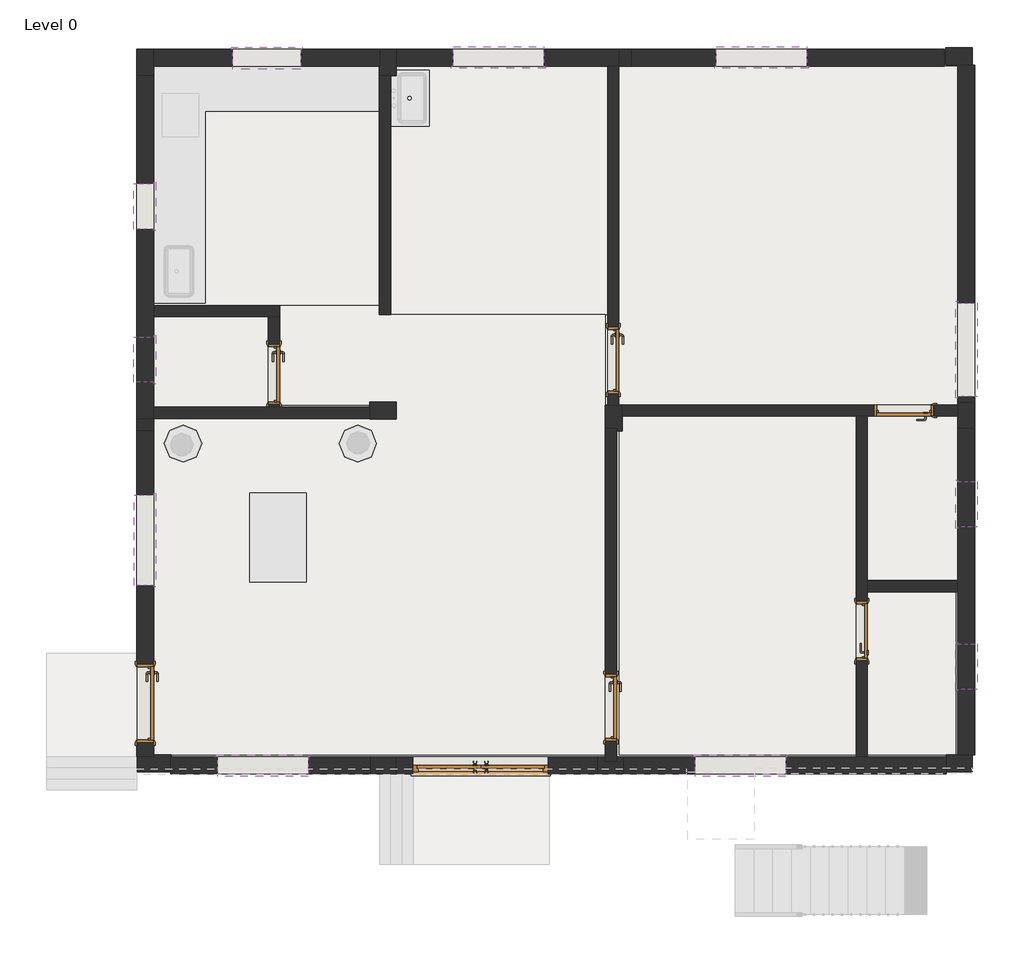
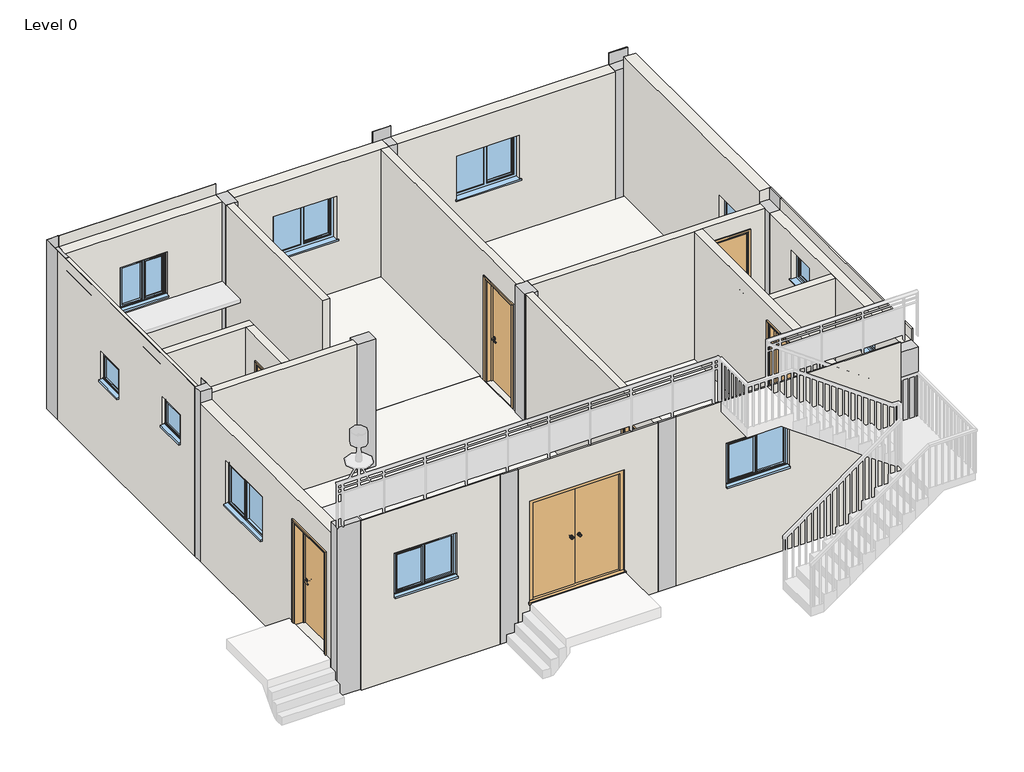
# One storey, part 1 of 3: 19 walls, 12 columns, 11 windows, 7 doors, 5 slabs.
# Revit data of these elements (continued)
# Type "Windows_Dbl_Plain : W3" (continued)
#   Height = 2.985564 ft
#   Width = 4.136 ft
#   Heat Transfer Coefficient (U) = 3.6886 W/(m²·K)
#   Glazing Thickness = 0.07874 ft
#   FrameOffset - External = 0.164042 ft
#   Frame Depth = 0.213255 ft
#   Default Head Height = 6.922572 ft
#   Cill Depth = 0.287073 ft
#   Cavity Closer Width = 0.164042 ft
#   Cavity Closer Offset from Ext = 0.336286 ft
#   Cavity Closer Depth = 0.278871 ft
#   Vis - Cavity Closers = yes
#   Define Thermal Properties by = 1
#   Material Trim = Window Frame
#   Material Glass = Glass
#   Material Frame = Cherry
#   Wall Closure = (empty or 0)
# Type "Windows_Dbl_Plain : W4"
#   Type Mark = "58"
#   Operation = "DoublePanelVertical"
#   Construction Type Id = "GSP4R"
#   Manufacturer = "Revit"
#   Keynote = "L10"
#   Analytic Construction = "1/8 in Pilkington single glazing"
#   Wrap Layers (Ext) from Ext = 0.336286 ft
#   Wrap Layers (Int) from Ext = 0.582349 ft
#   Window Board Projection = 0.082021 ft
#   Window Board Extension = 0.082021 ft
#   Visual Light Transmittance = 0.9
#   Solar Heat Gain Coefficient = 0.78
#   Rough Width = 4.0 ft
#   Rough Height = 2.985564 ft
#   Height = 2.985564 ft
#   Width = 4.0 ft
#   Heat Transfer Coefficient (U) = 3.6886 W/(m²·K)
#   Glazing Thickness = 0.07874 ft
#   FrameOffset - External = 0.164042 ft
#   Frame Depth = 0.213255 ft
#   Default Head Height = 6.922572 ft
#   Cill Depth = 0.287073 ft
#   Cavity Closer Width = 0.164042 ft
#   Cavity Closer Offset from Ext = 0.336286 ft
#   Cavity Closer Depth = 0.278871 ft
#   Vis - Cavity Closers = yes
#   Define Thermal Properties by = 1
#   Material Trim = Window Frame
#   Material Glass = Glass
#   Material Frame = Cherry
#   Wall Closure = (empty or 0)
# Type "Windows_Dbl_Plain : W5"
#   Type Mark = "57"
#   Operation = "DoublePanelVertical"
#   Construction Type Id = "GSP4R"
#   Manufacturer = "Revit"
#   Keynote = "L10"
#   Analytic Construction = "1/8 in Pilkington single glazing"
#   Wrap Layers (Ext) from Ext = 0.336286 ft
#   Wrap Layers (Int) from Ext = 0.582349 ft
#   Window Board Projection = 0.082021 ft
#   Window Board Extension = 0.082021 ft
#   Visual Light Transmittance = 0.9
#   Solar Heat Gain Coefficient = 0.78
#   Rough Width = 4.018 ft
#   Rough Height = 2.985564 ft
#   Height = 2.985564 ft
#   Width = 4.018 ft
#   Heat Transfer Coefficient (U) = 3.6886 W/(m²·K)
#   Glazing Thickness = 0.07874 ft
#   FrameOffset - External = 0.164042 ft
#   Frame Depth = 0.213255 ft
#   Default Head Height = 6.922572 ft
#   Cill Depth = 0.287073 ft
#   Cavity Closer Width = 0.164042 ft
#   Cavity Closer Offset from Ext = 0.336286 ft
#   Cavity Closer Depth = 0.278871 ft
#   Vis - Cavity Closers = yes
#   Define Thermal Properties by = 1
#   Material Trim = Window Frame
#   Material Glass = Glass
#   Material Frame = Cherry
#   Wall Closure = (empty or 0)
# Type "Windows_Dbl_Plain : W6"
#   Type Mark = "56"
#   Operation = "DoublePanelVertical"
#   Construction Type Id = "GSP4R"
#   Manufacturer = "Revit"
#   Keynote = "L10"
#   Analytic Construction = "1/8 in Pilkington single glazing"
#   Wrap Layers (Ext) from Ext = 0.336286 ft
#   Wrap Layers (Int) from Ext = 0.582349 ft
#   Window Board Projection = 0.082021 ft
#   Window Board Extension = 0.082021 ft
#   Visual Light Transmittance = 0.9
#   Solar Heat Gain Coefficient = 0.78
#   Rough Width = 3.0 ft
#   Rough Height = 2.985564 ft
#   Height = 2.985564 ft
#   Width = 3.0 ft
#   Heat Transfer Coefficient (U) = 3.6886 W/(m²·K)
#   Glazing Thickness = 0.07874 ft
#   FrameOffset - External = 0.164042 ft
#   Frame Depth = 0.213255 ft
#   Default Head Height = 6.922572 ft
#   Cill Depth = 0.287073 ft
#   Cavity Closer Width = 0.164042 ft
#   Cavity Closer Offset from Ext = 0.336286 ft
#   Cavity Closer Depth = 0.278871 ft
#   Vis - Cavity Closers = yes
#   Define Thermal Properties by = 1
#   Material Trim = Window Frame
#   Material Glass = Glass
#   Material Frame = Cherry
#   Wall Closure = (empty or 0)
# Type "Windows_Dbl_Plain : W7"
#   Type Mark = "63"
#   Operation = "DoublePanelVertical"
#   Construction Type Id = "GSP4R"
#   Manufacturer = "Revit"
#   Keynote = "L10"
#   Analytic Construction = "1/8 in Pilkington single glazing"
#   Wrap Layers (Ext) from Ext = 0.336286 ft
#   Wrap Layers (Int) from Ext = 0.582349 ft
#   Window Board Projection = 0.082021 ft
#   Window Board Extension = 0.082021 ft
#   Visual Light Transmittance = 0.9
#   Solar Heat Gain Coefficient = 0.78
#   Rough Width = 4.0 ft
#   Rough Height = 2.985564 ft
#   Height = 2.985564 ft
#   Width = 4.0 ft
#   Heat Transfer Coefficient (U) = 3.6886 W/(m²·K)
#   Glazing Thickness = 0.07874 ft
#   FrameOffset - External = 0.164042 ft
#   Frame Depth = 0.213255 ft
#   Default Head Height = 6.922572 ft
#   Cill Depth = 0.287073 ft
#   Cavity Closer Width = 0.164042 ft
#   Cavity Closer Offset from Ext = 0.336286 ft
#   Cavity Closer Depth = 0.278871 ft
#   Vis - Cavity Closers = yes
#   Define Thermal Properties by = 1
#   Material Trim = Window Frame
#   Material Glass = Glass
#   Material Frame = Cherry
#   Wall Closure = (empty or 0)
# Type "Windows_Dbl_Plain : WN"
#   Type Mark = "61"
#   Operation = "DoublePanelVertical"
#   Construction Type Id = "GSP4R"
#   Manufacturer = "Revit"
#   Keynote = "L10"
#   Analytic Construction = "1/8 in Pilkington single glazing"
#   Wrap Layers (Ext) from Ext = 0.336286 ft
#   Wrap Layers (Int) from Ext = 0.582349 ft
#   Window Board Projection = 0.082021 ft
#   Window Board Extension = 0.082021 ft
#   Visual Light Transmittance = 0.9
#   Solar Heat Gain Coefficient = 0.78
#   Rough Width = 4.0 ft
#   Rough Height = 2.985564 ft
#   Height = 2.985564 ft
#   Width = 4.0 ft
#   Heat Transfer Coefficient (U) = 3.6886 W/(m²·K)
#   Glazing Thickness = 0.07874 ft
#   FrameOffset - External = 0.164042 ft
#   Frame Depth = 0.213255 ft
#   Default Head Height = 6.922572 ft
#   Cill Depth = 0.287073 ft
#   Cavity Closer Width = 0.164042 ft
#   Cavity Closer Offset from Ext = 0.336286 ft
#   Cavity Closer Depth = 0.278871 ft
#   Vis - Cavity Closers = yes
#   Define Thermal Properties by = 1
#   Material Trim = Window Frame
#   Material Glass = Glass
#   Material Frame = Cherry
#   Wall Closure = (empty or 0)
# Type "Windows_Sgl_Plain : VW1"
#   Type Mark = "64"
#   Operation = "SinglePanel"
#   Construction Type Id = "SGL"
#   Manufacturer = "Revit"
#   Keynote = "L10"
#   Analytic Construction = "Large single-glazed windows"
#   Wrap Layers (Ext) from Ext = 0.336286 ft
#   Wrap Layers (Int) from Ext = 0.582349 ft
#   Window Board Projection = 0.082021 ft
#   Window Board Extension = 0.082021 ft
#   Visual Light Transmittance = 0.9
#   Solar Heat Gain Coefficient = 0.86
#   Rough Width = 2.0 ft
#   Rough Height = 2.0 ft
#   Height = 2.0 ft
#   Width = 2.0 ft
#   Heat Transfer Coefficient (U) = 5.5617 W/(m²·K)
#   Glazing Thickness = 0.07874 ft
#   FrameOffset - External = 0.164042 ft
#   Frame Depth = 0.213255 ft
#   Default Head Height = 6.922572 ft
#   Cill Depth = 0.287073 ft
#   Cavity Closer Width = 0.164042 ft
#   Cavity Closer Offset from Ext = 0.336286 ft
#   Cavity Closer Depth = 0.278871 ft
#   Vis - Cavity Closers = yes
#   Define Thermal Properties by = 1
#   Material Trim = Window Frame
#   Material Glass = Glass
#   Material Frame = Window Frame
#   Wall Closure = (empty or 0)
# Type "Windows_Sgl_Plain : VW2"
#   Type Mark = "65"
#   Operation = "SinglePanel"
#   Construction Type Id = "SGL"
#   Manufacturer = "Revit"
#   Keynote = "L10"
#   Analytic Construction = "Large single-glazed windows"
#   Wrap Layers (Ext) from Ext = 0.336286 ft
#   Wrap Layers (Int) from Ext = 0.582349 ft
#   Window Board Projection = 0.082021 ft
#   Window Board Extension = 0.082021 ft
#   Visual Light Transmittance = 0.9
#   Solar Heat Gain Coefficient = 0.86
#   Rough Width = 2.0 ft
#   Rough Height = 2.0 ft
#   Height = 2.0 ft
#   Width = 2.0 ft
#   Heat Transfer Coefficient (U) = 5.5617 W/(m²·K)
#   Glazing Thickness = 0.07874 ft
#   FrameOffset - External = 0.164042 ft
#   Frame Depth = 0.213255 ft
#   Default Head Height = 6.922572 ft
#   Cill Depth = 0.287073 ft
#   Cavity Closer Width = 0.164042 ft
#   Cavity Closer Offset from Ext = 0.336286 ft
#   Cavity Closer Depth = 0.278871 ft
#   Vis - Cavity Closers = yes
#   Define Thermal Properties by = 1
#   Material Trim = Window Frame
#   Material Glass = Glass
#   Material Frame = Window Frame
#   Wall Closure = (empty or 0)
# Type "Windows_Sgl_Plain : VW3"
#   Type Mark = "44"
#   Operation = "SinglePanel"
#   Construction Type Id = "SGL"
#   Manufacturer = "Revit"
#   Keynote = "L10"
#   Analytic Construction = "Large single-glazed windows"
#   Wrap Layers (Ext) from Ext = 0.336286 ft
#   Wrap Layers (Int) from Ext = 0.582349 ft
#   Window Board Projection = 0.082021 ft
#   Window Board Extension = 0.082021 ft
#   Visual Light Transmittance = 0.9
#   Solar Heat Gain Coefficient = 0.86
#   Rough Width = 2.0 ft
#   Rough Height = 2.0 ft
#   Height = 2.0 ft
#   Width = 2.0 ft
#   Heat Transfer Coefficient (U) = 5.5617 W/(m²·K)
#   Glazing Thickness = 0.07874 ft
#   FrameOffset - External = 0.164042 ft
#   Frame Depth = 0.213255 ft
#   Default Head Height = 6.922572 ft
#   Cill Depth = 0.287073 ft
#   Cavity Closer Width = 0.164042 ft
#   Cavity Closer Offset from Ext = 0.336286 ft
#   Cavity Closer Depth = 0.278871 ft
#   Vis - Cavity Closers = yes
#   Define Thermal Properties by = 1
#   Material Trim = Window Frame
#   Material Glass = Glass
#   Material Frame = Window Frame
#   Wall Closure = (empty or 0)
# Type "Windows_Sgl_Plain : VW4"
#   Type Mark = "60"
#   Operation = "SinglePanel"
#   Construction Type Id = "SGL"
#   Manufacturer = "Revit"
#   Keynote = "L10"
#   Analytic Construction = "Large single-glazed windows"
#   Wrap Layers (Ext) from Ext = 0.336286 ft
#   Wrap Layers (Int) from Ext = 0.582349 ft
#   Window Board Projection = 0.082021 ft
#   Window Board Extension = 0.082021 ft
#   Visual Light Transmittance = 0.9
#   Solar Heat Gain Coefficient = 0.86
#   Rough Width = 2.0 ft
#   Rough Height = 2.0 ft
#   Height = 2.0 ft
#   Width = 2.0 ft
#   Heat Transfer Coefficient (U) = 5.5617 W/(m²·K)
#   Glazing Thickness = 0.07874 ft
#   FrameOffset - External = 0.164042 ft
#   Frame Depth = 0.213255 ft
#   Default Head Height = 6.922572 ft
#   Cill Depth = 0.287073 ft
#   Cavity Closer Width = 0.164042 ft
#   Cavity Closer Offset from Ext = 0.336286 ft
#   Cavity Closer Depth = 0.278871 ft
#   Vis - Cavity Closers = yes
#   Define Thermal Properties by = 1
#   Material Trim = Window Frame
#   Material Glass = Glass
#   Material Frame = Window Frame
#   Wall Closure = (empty or 0)
# Elements 1, 2, 3, 4, 5, 6, 7, 8, 9 (IfcColumn, "Columns_Rectangular : C1")
#   Phase Created = New Construction
#   Materials on its faces: "Concrete, Precast"
# Elements 10, 11, 12 (IfcColumn, "Columns_Rectangular : C2")
#   Phase Created = New Construction
#   Materials on its faces: "Concrete, Precast"
# Element 13 (IfcDoor, "Doors_ExtDbl_Flush : D1")
#   Phase Created = New Construction
#   Materials on its faces: "Door - Handle", "Door - Frame/Mullion", "Door - Panel"
# Element 14 (IfcDoor, "Doors_IntSgl : D2")
#   Phase Created = New Construction
#   Materials on its faces: "Door - Architrave", "Door - Handle", "Door - Frame/Mullion (1)", "Door - Panel"
# Element 15 (IfcDoor, "Doors_IntSgl : D3")
#   Phase Created = New Construction
#   Materials on its faces: "Door - Architrave", "Door - Handle", "Door - Frame/Mullion (1)", "Door - Panel"
# Element 16 (IfcDoor, "Doors_IntSgl : D4")
#   Phase Created = New Construction
#   Materials on its faces: "Door - Architrave", "Door - Handle", "Door - Frame/Mullion (1)", "Door - Panel"
# Element 17 (IfcDoor, "Doors_IntSgl : D5")
#   Phase Created = New Construction
#   Materials on its faces: "Door - Architrave", "Door - Handle", "Door - Frame/Mullion (1)", "Door - Panel"
# Element 18 (IfcDoor, "Doors_IntSgl : D6")
#   Phase Created = New Construction
#   Materials on its faces: "Door - Architrave", "Door - Handle", "Door - Frame/Mullion (1)", "Door - Panel"
# Element 19 (IfcDoor, "Doors_IntSgl : D7")
#   Phase Created = New Construction
#   Materials on its faces: "Door - Architrave", "Door - Handle", "Door - Frame/Mullion (1)", "Door - Panel"
# Element 20 (IfcSlab)
#   Height Offset From Level = 0.492 ft
#   Phase Created = New Construction
#   Materials on its faces: "Structure, Timber Joist/Rafter Layer"
# Element 21 (IfcSlab, "BEDROOM FLOOR")
#   Height Offset From Level = 0.492 ft
#   Phase Created = New Construction
#   Materials on its faces: "Structure, Timber Joist/Rafter Layer", "BEDROOM FLOOR TEXTURE"
# Element 22 (IfcSlab, "KITCHEN FLOOR")
#   Height Offset From Level = 0.492 ft
#   Phase Created = New Construction
#   Materials on its faces: "Structure, Timber Joist/Rafter Layer", "KITCHEN FLOOR TEXTURE"
# Element 23 (IfcSlab, "LIVING ROOM")
#   built-in parameter 1001955 = 3.14159 (stored number, unit not read)
#   Height Offset From Level = 0.492 ft
#   Phase Created = New Construction
#   Materials on its faces: "Structure, Timber Joist/Rafter Layer", "LIVING ROOM FLOOR TEXTURE"
# Element 24 (IfcSlab, "TOILET FLOOR")
#   built-in parameter 1001955 = 3.14159 (stored number, unit not read)
#   Height Offset From Level = 0.984 ft
#   Phase Created = New Construction
#   Materials on its faces: "Structure, Timber Joist/Rafter Layer", "TOILET FLOOR TEXTURE"
# Elements 25, 26, 27, 28, 29, 30, 31, 32, 33, 34 (IfcWall, "EX WALL")
#   built-in parameter 1001111 = -1.551 ft
#   Top Offset = 0.0 ft
#   Base Offset = -1.551 ft
#   wall height = 11.39352 ft
#   Phase Created = New Construction
#   Base Constraint = Level 0
#   Top Constraint = Level 1
#   Materials on its faces: "Brick, Common"
# Elements 35, 36, 37, 38, 39, 40, 41, 42, 43 (IfcWall, "INNER WALL")
#   Top Offset = 0.0 ft
#   Base Offset = 0.0 ft
#   wall height = 9.84252 ft
#   Phase Created = New Construction
#   Base Constraint = Level 0
#   Top Constraint = Level 1
#   Materials on its faces: "Brick, Common"
# Element 44 (IfcWindow, "Windows_Dbl_Plain : W1")
#   Mark = "W1"
#   Phase Created = New Construction
#   Materials on its faces: "Cherry", "Glass", "Window Frame"
# Element 45 (IfcWindow, "Windows_Dbl_Plain : W3")
#   Mark = "W3"
#   Phase Created = New Construction
#   Materials on its faces: "Cherry", "Glass", "Window Frame"
# Element 46 (IfcWindow, "Windows_Dbl_Plain : W4")
#   Mark = "W4"
#   Phase Created = New Construction
#   Materials on its faces: "Cherry", "Glass", "Window Frame"
# Element 47 (IfcWindow, "Windows_Dbl_Plain : W5")
#   Mark = "W5"
#   Phase Created = New Construction
#   Materials on its faces: "Cherry", "Glass", "Window Frame"
# Element 48 (IfcWindow, "Windows_Dbl_Plain : W6")
#   Mark = "W6"
#   Phase Created = New Construction
#   Materials on its faces: "Cherry", "Glass", "Window Frame"
# Element 49 (IfcWindow, "Windows_Dbl_Plain : W7")
#   Mark = "W7"
#   Phase Created = New Construction
#   Materials on its faces: "Cherry", "Glass", "Window Frame"
# Element 50 (IfcWindow, "Windows_Dbl_Plain : WN")
#   Mark = "W2"
#   Phase Created = New Construction
#   Materials on its faces: "Cherry", "Glass", "Window Frame"
# Element 51 (IfcWindow, "Windows_Sgl_Plain : VW1")
#   Mark = "VW1"
#   Phase Created = New Construction
#   Materials on its faces: "Window Frame", "Glass"
# Element 52 (IfcWindow, "Windows_Sgl_Plain : VW2")
#   Mark = "VW2"
#   Phase Created = New Construction
#   Materials on its faces: "Window Frame", "Glass"
# Element 53 (IfcWindow, "Windows_Sgl_Plain : VW3")
#   Mark = "VW3"
#   Phase Created = New Construction
#   Materials on its faces: "Window Frame", "Glass"
# Element 54 (IfcWindow, "Windows_Sgl_Plain : VW4")
#   Mark = "VW4"
#   Phase Created = New Construction
#   Materials on its faces: "Window Frame", "Glass"
# Materials
#   "Concrete, Precast": class "Concrete", colour RGB 192 192 192, transparency 0, Description = "Precast concrete", Cost = 0
#   "Door - Panel": class "Wood", colour RGB 210 159 95, transparency 0, Keynote = "L20", Cost = 0
#   "Door - Frame/Mullion": class "Wood", colour RGB 212 179 113, transparency 0, Keynote = "L20", Cost = 0
#   "Door - Handle": colour RGB 0 0 0, transparency 0, Keynote = "P21", Cost = 0
#   "Door - Frame/Mullion (1)": class "Wood", colour RGB 212 179 113, transparency 0, Keynote = "L20", Cost = 0
#   "Door - Architrave": class "Wood", colour RGB 154 90 5, transparency 0, Keynote = "P20", Cost = 0
#   "BEDROOM FLOOR TEXTURE": class "Generic", colour RGB 120 120 120, transparency 0, Cost = 0
#   "Structure, Timber Joist/Rafter Layer": class "Wood", colour RGB 127 127 127, transparency 0, Description = "Timber framing, thermal airspace", Cost = 0
#   "KITCHEN FLOOR TEXTURE": class "Generic", colour RGB 120 120 120, transparency 0, Cost = 0
#   "LIVING ROOM FLOOR TEXTURE": class "Generic", colour RGB 120 120 120, transparency 0, Cost = 0
#   "TOILET FLOOR TEXTURE": class "Generic", colour RGB 120 120 120, transparency 0, Cost = 0
#   "Brick, Common": class "Masonry", colour RGB 170 100 105, transparency 0, Description = "Common brick", Cost = 0
#   "Window Frame": colour RGB 249 249 249, transparency 0, Keynote = "L10", Cost = 0
#   "Glass": class "Glass", colour RGB 0 128 192, transparency 0.9, Description = "Soda Lime Glass", Cost = 0
#   "Cherry": class "Wood", colour RGB 226 177 128, transparency 0, Description = "Prunus Serotina", Cost = 0
